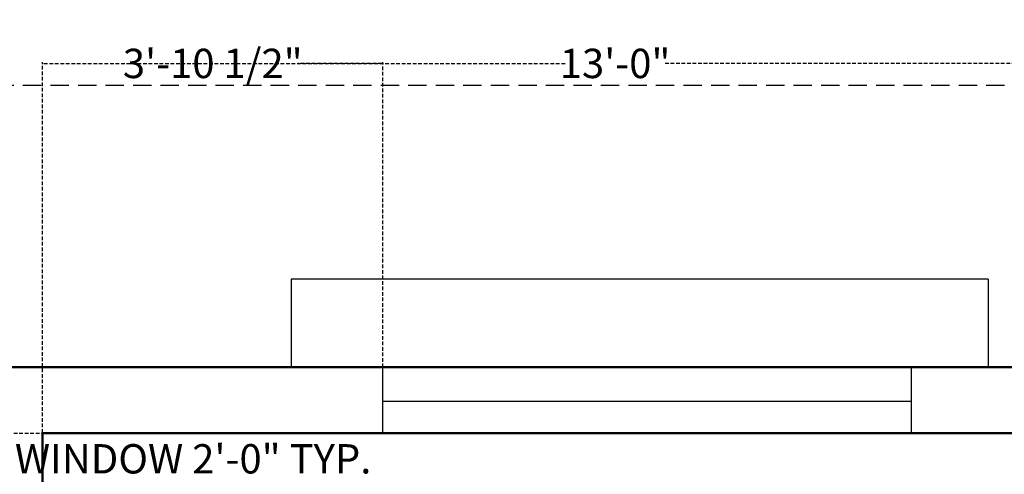
# Model space of a CAD drawing. Units: inches. Extents: x 513 to 1142, y 396 to 927.
# Tile 30 of 31: x 922 to 1056, y 865 to 927. Entities that reach past the tile are written whole.
import ezdxf

# ---------------------------------------------------------------- set-up
doc = ezdxf.new("R2010")
doc.units = ezdxf.units.IN
doc.header["$MEASUREMENT"] = 0
doc.linetypes.add('DASHED', pattern=[0.75, 0.5, -0.25])
for name, color, linetype, lineweight in [('A-ANNO-DIMS', 2, 'DASHED', 18), ('A-WALL', 7, 'Continuous', 50), ('windows', 172, 'Continuous', 25)]:
    doc.layers.add(name, color=color, linetype=linetype, lineweight=lineweight)
doc.styles.get("Standard").update_dxf_attribs({"font": 'arial.ttf'})
doc.dimstyles.get("Standard").update_dxf_attribs({"dimtxt": 4, "dimasz": 0.18, "dimexe": 0.18, "dimexo": 0.0625, "dimgap": 0.09, "dimtad": 0, "dimtih": 1, "dimtoh": 1, "dimdec": 0, "dimrnd": 6, "dimzin": 0, "dimdsep": 46, "dimlunit": 3, "dimtxsty": 'Standard', "dimcen": 0.09, "dimadec": 0, "dimazin": 0, "dimtfac": 1, "dimtdec": 0, "dimtofl": 0, "dimtmove": 0, "dimatfit": 3, "dimfxl": 1, "dimtolj": 1, "dimtzin": 0, "dimarcsym": 0})

# ---------------------------------------------------------------- blocks, each defined once
blk = doc.blocks.new('*D103')
at = {"layer": 'A-ANNO-DIMS', "color": 0, "lineweight": -2, "ltscale": 5, "transparency": 16777216}
for p, q in [((575, 879.22), (575, 917.74)), ((1090, 879.22), (1090, 917.74)), ((575.18, 917.56), (828.93, 917.56)), ((1089.82, 917.56), (836.06, 917.56))]:
    blk.add_line(p, q, dxfattribs=at)
at = {"layer": 'A-ANNO-DIMS', "color": 0, "ltscale": 5, "transparency": 16777216}
for points in [[(575.18, 917.59), (575.18, 917.53), (575, 917.56)], [(1089.82, 917.59), (1089.82, 917.53), (1090, 917.56)]]:
    blk.add_solid(points, dxfattribs=at)
at = {"layer": 'Defpoints', "color": 0, "ltscale": 5, "transparency": 16777216}
for p in [(1090, 917.56), (575, 879.16), (1090, 879.16)]:
    blk.add_point(p, dxfattribs=at)
at = {"layer": 'A-ANNO-DIMS', "color": 0, "ltscale": 5, "transparency": 16777216, "insert": (832.5, 917.56), "char_height": 4, "attachment_point": 5}
blk.add_mtext("\\A1;43'", dxfattribs=at)
blk = doc.blocks.new('WIN-72IN')
blk.add_line((0, 4.45), (72, 4.45))
blk.add_lwpolyline([(72, 9), (72, 0), (0, 0), (0, 9)], close=True)
blk = doc.blocks.new('*D129')
at = {"layer": 'A-ANNO-DIMS', "color": 0, "lineweight": -2, "transparency": 16777216}
for p, q in [((870.48, 870.2), (870.48, 866.48)), ((894.48, 870.2), (894.48, 866.48)), ((870.66, 866.66), (894.3, 866.66)), ((894.48, 866.66), (894.66, 866.66))]:
    blk.add_line(p, q, dxfattribs=at)
at = {"layer": 'A-ANNO-DIMS', "color": 0, "transparency": 16777216}
for points in [[(870.66, 866.69), (870.66, 866.63), (870.48, 866.66)], [(894.3, 866.69), (894.3, 866.63), (894.48, 866.66)]]:
    blk.add_solid(points, dxfattribs=at)
at = {"layer": 'Defpoints', "color": 0, "transparency": 16777216}
for p in [(870.48, 870.26), (894.48, 870.26), (894.48, 866.66)]:
    blk.add_point(p, dxfattribs=at)
at = {"layer": 'A-ANNO-DIMS', "color": 0, "transparency": 16777216, "insert": (933.38, 866.66), "char_height": 4, "attachment_point": 5}
blk.add_mtext('\\A1;NARROW WINDOW 2\'-0" TYP.', dxfattribs=at)
blk = doc.blocks.new('*D138')
at = {"layer": 'A-ANNO-DIMS', "color": 0, "lineweight": -2, "transparency": 16777216}
for p, q in [((925, 870.22), (925, 920.74)), ((925.18, 920.56), (996.22, 920.56)), ((1080.82, 920.56), (1009.77, 920.56)), ((1081, 870.22), (1081, 920.74))]:
    blk.add_line(p, q, dxfattribs=at)
at = {"layer": 'A-ANNO-DIMS', "color": 0, "transparency": 16777216}
for points in [[(925.18, 920.59), (925.18, 920.53), (925, 920.56)], [(1080.82, 920.59), (1080.82, 920.53), (1081, 920.56)]]:
    blk.add_solid(points, dxfattribs=at)
at = {"layer": 'Defpoints', "color": 0, "transparency": 16777216}
for p in [(1081, 920.56), (925, 870.16), (1081, 870.16)]:
    blk.add_point(p, dxfattribs=at)
at = {"layer": 'A-ANNO-DIMS', "color": 0, "transparency": 16777216, "insert": (1003, 920.56), "char_height": 4, "attachment_point": 5}
blk.add_mtext('\\A1;13\'-0"', dxfattribs=at)
blk = doc.blocks.new('*D148')
at = {"layer": 'A-ANNO-DIMS', "color": 0, "lineweight": -2, "transparency": 16777216}
for p, q in [((921.06, 870.16), (1131.58, 870.16)), ((1131.4, 869.98), (1131.4, 824.29)), ((1131.4, 774.34), (1131.4, 820.03)), ((897.06, 774.16), (1131.58, 774.16))]:
    blk.add_line(p, q, dxfattribs=at)
at = {"layer": 'A-ANNO-DIMS', "color": 0, "transparency": 16777216}
for points in [[(1131.37, 869.98), (1131.43, 869.98), (1131.4, 870.16)], [(1131.37, 774.34), (1131.43, 774.34), (1131.4, 774.16)]]:
    blk.add_solid(points, dxfattribs=at)
at = {"layer": 'Defpoints', "color": 0, "transparency": 16777216}
for p in [(921, 870.16), (1131.4, 870.16), (897, 774.16)]:
    blk.add_point(p, dxfattribs=at)
at = {"layer": 'A-ANNO-DIMS', "color": 0, "transparency": 16777216, "insert": (1131.4, 822.16), "char_height": 4, "attachment_point": 5}
blk.add_mtext('\\A1;8\'-0"', dxfattribs=at)
blk = doc.blocks.new('*D155')
at = {"layer": 'A-ANNO-DIMS', "color": 0, "lineweight": -2, "transparency": 16777216}
for p, q in [((925, 870.22), (925, 920.74)), ((925.18, 920.56), (936.56, 920.56)), ((971.18, 920.56), (959.8, 920.56)), ((971.36, 870.15), (971.36, 920.74))]:
    blk.add_line(p, q, dxfattribs=at)
at = {"layer": 'A-ANNO-DIMS', "color": 0, "transparency": 16777216}
for points in [[(925.18, 920.59), (925.18, 920.53), (925, 920.56)], [(971.18, 920.59), (971.18, 920.53), (971.36, 920.56)]]:
    blk.add_solid(points, dxfattribs=at)
at = {"layer": 'Defpoints', "color": 0, "transparency": 16777216}
for p in [(971.36, 920.56), (925, 870.16), (971.36, 870.09)]:
    blk.add_point(p, dxfattribs=at)
at = {"layer": 'A-ANNO-DIMS', "color": 0, "transparency": 16777216, "insert": (948.18, 920.56), "char_height": 4, "attachment_point": 5}
blk.add_mtext('\\A1;3\'-10 1/2"', dxfattribs=at)

msp = doc.modelspace()

# ---------------------------------------------------------------- linework, layer by layer
at = {"layer": 'A-WALL'}
for p, q in [((1090, 879.16), (575, 879.16)), ((1081, 870.16), (925, 870.16)), ((925, 770.16), (925, 870.16))]:
    msp.add_line(p, q, dxfattribs=at)
at = {"layer": 'windows'}
for p, q in [((1053.84, 891.16), (958.85, 891.16)), ((958.85, 891.16), (958.85, 879.16)), ((1053.84, 891.16), (1053.84, 879.16))]:
    msp.add_line(p, q, dxfattribs=at)

# ---------------------------------------------------------------- block references
msp.add_blockref('WIN-72IN', (971.36, 870.09), dxfattribs=at)

# ---------------------------------------------------------------- dimensions: what is measured, and where the dimension line sits
at = {"layer": 'A-ANNO-DIMS'}
for base, p2, picture, middle in [((971.36, 920.56), (971.36, 870.09), '*D155', (948.18, 920.56)), ((1081, 920.56), (1081, 870.16), '*D138', (1003, 920.56))]:
    dim = msp.add_linear_dim(base=base, p1=(925, 870.16), p2=p2, dimstyle='Standard', override={"dimdec": 1, "dimlfac": 1, "dimrnd": 0, "dimzin": 1, "dimdsep": 46, "dimlunit": 4, "dimfrac": 2}, dxfattribs=at)
    dim.commit()
    dim.dimension.update_dxf_attribs({"geometry": picture, "text_midpoint": middle})
at = {"layer": 'A-ANNO-DIMS', "ltscale": 5}
dim = msp.add_linear_dim(base=(1090, 917.56), p1=(575, 879.16), p2=(1090, 879.16), dimstyle='Standard', override={"dimclrd": 0, "dimclre": 0, "dimclrt": 0}, dxfattribs=at)
dim.commit()
dim.dimension.update_dxf_attribs({"geometry": '*D103', "text_midpoint": (832.5, 917.56)})
at = {"layer": 'A-ANNO-DIMS'}
dim = msp.add_linear_dim(base=(894.48, 866.66), p1=(870.48, 870.26), p2=(894.48, 870.26), text='NARROW WINDOW <> TYP.', dimstyle='Standard', override={"dimdec": 1, "dimlfac": 1, "dimrnd": 0, "dimzin": 1, "dimdsep": 46, "dimlunit": 4, "dimfrac": 2}, dxfattribs=at)
dim.commit()
dim.dimension.update_dxf_attribs({"geometry": '*D129', "text_midpoint": (933.38, 866.66)})
dim = msp.add_linear_dim(base=(1131.4, 870.16), p1=(897, 774.16), p2=(921, 870.16), angle=90, dimstyle='Standard', override={"dimdec": 1, "dimlfac": 1, "dimrnd": 0, "dimzin": 1, "dimdsep": 46, "dimlunit": 4, "dimfrac": 2}, dxfattribs=at)
dim.commit()
dim.dimension.update_dxf_attribs({"geometry": '*D148', "text_midpoint": (1131.4, 822.16)})

doc.saveas('drawing.dxf')
